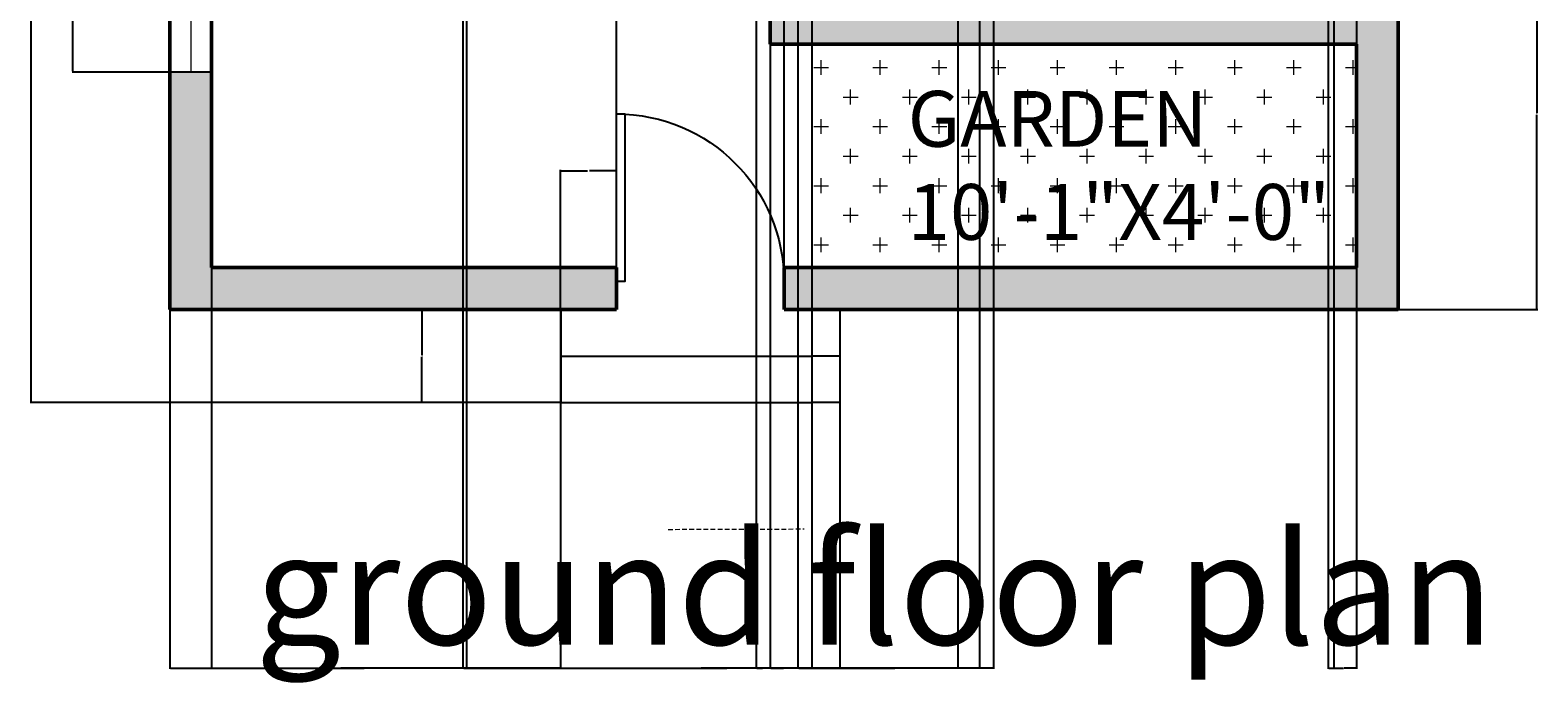
# Model space of a CAD drawing. Units: inches. Extents: x 1489 to 1813, y 1703 to 2293.
# Tile 1 of 4: x 1489 to 1813, y 1703 to 1843. Entities that reach past the tile are written whole.
import ezdxf

# ---------------------------------------------------------------- set-up
doc = ezdxf.new("R2010")
doc.units = ezdxf.units.IN
doc.header["$LTSCALE"] = 0.4
doc.linetypes.add('HIDDEN', pattern=[9.525, 6.35, -3.175])
for name, color, linetype, lineweight in [('A-ANNO-DIMS', 2, 'Continuous', 18), ('A-ANNO-HIDN', 7, 'HIDDEN', 18), ('A-ANNO-TEXT', 7, 'Continuous', 35), ('A-AREA-IDEN', 7, 'Continuous', 18), ('A-DOOR', 4, 'Continuous', 25), ('A-FLOR-STRS', 7, 'Continuous', 25), ('A-GLAZ', 4, 'Continuous', 18), ('A-WALL', 7, 'Continuous', 50), ('L-PLNT', 3, 'Continuous', 18)]:
    doc.layers.add(name, color=color, linetype=linetype, lineweight=lineweight)
doc.layers.add('A-WALL-PATT', color=18, linetype='HIDDEN', lineweight=13, true_color=0x000000)
doc.layers.add('L-PLNT-PATT', color=114, linetype='Continuous', lineweight=13, true_color=0x139b48)
doc.styles.get("Standard").update_dxf_attribs({"font": 'arial.ttf'})
doc.dimstyles.get("Standard").update_dxf_attribs({"dimtxt": 0.18, "dimasz": 0.18, "dimexe": 0.18, "dimexo": 0.0625, "dimgap": 0.09, "dimtad": 0, "dimtih": 1, "dimtoh": 1, "dimdec": 4, "dimzin": 0, "dimdsep": 46, "dimtxsty": 'Standard', "dimcen": 0.09, "dimadec": 0, "dimazin": 0, "dimtfac": 1, "dimtdec": 4, "dimtofl": 0, "dimtmove": 0, "dimatfit": 3, "dimfxl": 1, "dimtolj": 1, "dimtzin": 0, "dimarcsym": 0})

# ---------------------------------------------------------------- blocks, each defined once
blk = doc.blocks.new('*U5')
for p, q in [((-36, 0), (-36, -6)), ((0, 0), (0, -6))]:
    blk.add_line(p, q)
blk.add_lwpolyline([(0, 0), (0, 36), (-1.75, 36), (-1.75, 0)], close=True)
blk.add_arc((0, 0), 36, 90, 180)
blk = doc.blocks.new('*D29')
at = {"layer": 'A-ANNO-DIMS', "color": 0, "lineweight": -2, "ltscale": 0.4, "transparency": 16777216}
for p, q in [((1518.92, 2263.17), (1489, 2263.17)), ((1489.18, 2262.99), (1489.18, 2013.35)), ((1489.18, 1763.35), (1489.18, 2012.99)), ((1602.92, 1763.17), (1489, 1763.17))]:
    blk.add_line(p, q, dxfattribs=at)
at = {"layer": 'A-ANNO-DIMS', "color": 0, "ltscale": 0.4, "transparency": 16777216}
for points in [[(1489.15, 2262.99), (1489.21, 2262.99), (1489.18, 2263.17)], [(1489.15, 1763.35), (1489.21, 1763.35), (1489.18, 1763.17)]]:
    blk.add_solid(points, dxfattribs=at)
at = {"layer": 'Defpoints', "color": 0, "ltscale": 0.4, "transparency": 16777216}
for p in [(1489.18, 2263.17), (1518.98, 2263.17), (1602.98, 1763.17)]:
    blk.add_point(p, dxfattribs=at)
at = {"layer": 'A-ANNO-DIMS', "color": 0, "ltscale": 0.4, "transparency": 16777216, "insert": (1489.18, 2013.17), "char_height": 0.18, "attachment_point": 5}
blk.add_mtext('\\A1;500', dxfattribs=at)
blk = doc.blocks.new('*D30')
at = {"layer": 'A-ANNO-DIMS', "color": 0, "lineweight": -2, "ltscale": 0.4, "transparency": 16777216}
for p, q in [((1518.98, 1783.11), (1518.98, 1705.95)), ((1602.98, 1783.11), (1602.98, 1705.95)), ((1519.16, 1706.13), (1560.77, 1706.13)), ((1602.8, 1706.13), (1561.2, 1706.13))]:
    blk.add_line(p, q, dxfattribs=at)
at = {"layer": 'A-ANNO-DIMS', "color": 0, "ltscale": 0.4, "transparency": 16777216}
for points in [[(1519.16, 1706.16), (1519.16, 1706.1), (1518.98, 1706.13)], [(1602.8, 1706.16), (1602.8, 1706.1), (1602.98, 1706.13)]]:
    blk.add_solid(points, dxfattribs=at)
at = {"layer": 'Defpoints', "color": 0, "ltscale": 0.4, "transparency": 16777216}
for p in [(1518.98, 1783.17), (1602.98, 1783.17), (1602.98, 1706.13)]:
    blk.add_point(p, dxfattribs=at)
at = {"layer": 'A-ANNO-DIMS', "color": 0, "ltscale": 0.4, "transparency": 16777216, "insert": (1560.98, 1706.13), "char_height": 0.18, "attachment_point": 5}
blk.add_mtext('\\A1;84', dxfattribs=at)
blk = doc.blocks.new('*D31')
at = {"layer": 'A-ANNO-DIMS', "color": 0, "lineweight": -2, "ltscale": 0.4, "transparency": 16777216}
for p, q in [((1602.98, 1763.11), (1602.98, 1705.95)), ((1662.98, 1763.11), (1662.98, 1705.95)), ((1603.16, 1706.13), (1632.76, 1706.13)), ((1662.8, 1706.13), (1633.2, 1706.13))]:
    blk.add_line(p, q, dxfattribs=at)
at = {"layer": 'A-ANNO-DIMS', "color": 0, "ltscale": 0.4, "transparency": 16777216}
for points in [[(1603.16, 1706.16), (1603.16, 1706.1), (1602.98, 1706.13)], [(1662.8, 1706.16), (1662.8, 1706.1), (1662.98, 1706.13)]]:
    blk.add_solid(points, dxfattribs=at)
at = {"layer": 'Defpoints', "color": 0, "ltscale": 0.4, "transparency": 16777216}
for p in [(1602.98, 1763.17), (1662.98, 1763.17), (1662.98, 1706.13)]:
    blk.add_point(p, dxfattribs=at)
at = {"layer": 'A-ANNO-DIMS', "color": 0, "ltscale": 0.4, "transparency": 16777216, "insert": (1632.98, 1706.13), "char_height": 0.18, "attachment_point": 5}
blk.add_mtext('\\A1;60', dxfattribs=at)
blk = doc.blocks.new('*D32')
at = {"layer": 'A-ANNO-DIMS', "color": 0, "lineweight": -2, "ltscale": 0.4, "transparency": 16777216}
for p, q in [((1602.92, 1783.17), (1573, 1783.17)), ((1573.18, 1782.99), (1573.18, 1773.35)), ((1573.18, 1763.35), (1573.18, 1772.99)), ((1602.92, 1763.17), (1573, 1763.17))]:
    blk.add_line(p, q, dxfattribs=at)
at = {"layer": 'A-ANNO-DIMS', "color": 0, "ltscale": 0.4, "transparency": 16777216}
for points in [[(1573.15, 1782.99), (1573.21, 1782.99), (1573.18, 1783.17)], [(1573.15, 1763.35), (1573.21, 1763.35), (1573.18, 1763.17)]]:
    blk.add_solid(points, dxfattribs=at)
at = {"layer": 'Defpoints', "color": 0, "ltscale": 0.4, "transparency": 16777216}
for p in [(1573.18, 1783.17), (1602.98, 1783.17), (1602.98, 1763.17)]:
    blk.add_point(p, dxfattribs=at)
at = {"layer": 'A-ANNO-DIMS', "color": 0, "ltscale": 0.4, "transparency": 16777216, "insert": (1573.18, 1773.17), "char_height": 0.18, "attachment_point": 5}
blk.add_mtext('\\A1;20', dxfattribs=at)
blk = doc.blocks.new('*D33')
at = {"layer": 'A-ANNO-DIMS', "color": 0, "lineweight": -2, "ltscale": 0.4, "transparency": 16777216}
for p, q in [((1614.98, 1783.23), (1614.98, 2293.15)), ((1615.16, 2292.97), (1632.77, 2292.97)), ((1650.8, 2292.97), (1633.2, 2292.97)), ((1650.98, 1783.23), (1650.98, 2293.15))]:
    blk.add_line(p, q, dxfattribs=at)
at = {"layer": 'A-ANNO-DIMS', "color": 0, "ltscale": 0.4, "transparency": 16777216}
for points in [[(1615.16, 2293), (1615.16, 2292.94), (1614.98, 2292.97)], [(1650.8, 2293), (1650.8, 2292.94), (1650.98, 2292.97)]]:
    blk.add_solid(points, dxfattribs=at)
at = {"layer": 'Defpoints', "color": 0, "ltscale": 0.4, "transparency": 16777216}
for p in [(1650.98, 2292.97), (1614.98, 1783.17), (1650.98, 1783.17)]:
    blk.add_point(p, dxfattribs=at)
at = {"layer": 'A-ANNO-DIMS', "color": 0, "ltscale": 0.4, "transparency": 16777216, "insert": (1632.98, 2292.97), "char_height": 0.18, "attachment_point": 5}
blk.add_mtext('\\A1;36', dxfattribs=at)
blk = doc.blocks.new('*D34')
at = {"layer": 'A-ANNO-DIMS', "color": 0, "lineweight": -2, "ltscale": 0.4, "transparency": 16777216}
for p, q in [((1783.05, 1867.17), (1812.96, 1867.17)), ((1812.78, 1866.99), (1812.78, 1825.35)), ((1812.78, 1783.35), (1812.78, 1824.99)), ((1783.05, 1783.17), (1812.96, 1783.17))]:
    blk.add_line(p, q, dxfattribs=at)
at = {"layer": 'A-ANNO-DIMS', "color": 0, "ltscale": 0.4, "transparency": 16777216}
for points in [[(1812.75, 1866.99), (1812.81, 1866.99), (1812.78, 1867.17)], [(1812.75, 1783.35), (1812.81, 1783.35), (1812.78, 1783.17)]]:
    blk.add_solid(points, dxfattribs=at)
at = {"layer": 'Defpoints', "color": 0, "ltscale": 0.4, "transparency": 16777216}
for p in [(1782.98, 1867.17), (1812.78, 1867.17), (1782.98, 1783.17)]:
    blk.add_point(p, dxfattribs=at)
at = {"layer": 'A-ANNO-DIMS', "color": 0, "ltscale": 0.4, "transparency": 16777216, "insert": (1812.78, 1825.17), "char_height": 0.18, "attachment_point": 5}
blk.add_mtext('\\A1;84', dxfattribs=at)
blk = doc.blocks.new('*D41')
at = {"layer": 'A-ANNO-DIMS', "color": 0, "lineweight": -2, "ltscale": 0.4, "transparency": 16777216}
for p, q in [((1647.98, 2254.11), (1647.98, 1705.95)), ((1653.98, 2254.11), (1653.98, 1705.95)), ((1648.16, 1706.13), (1650.83, 1706.13)), ((1653.8, 1706.13), (1651.13, 1706.13))]:
    blk.add_line(p, q, dxfattribs=at)
at = {"layer": 'A-ANNO-DIMS', "color": 0, "ltscale": 0.4, "transparency": 16777216}
for points in [[(1648.16, 1706.16), (1648.16, 1706.1), (1647.98, 1706.13)], [(1653.8, 1706.16), (1653.8, 1706.1), (1653.98, 1706.13)]]:
    blk.add_solid(points, dxfattribs=at)
at = {"layer": 'Defpoints', "color": 0, "ltscale": 0.4, "transparency": 16777216}
for p in [(1647.98, 2254.17), (1653.98, 2254.17), (1653.98, 1706.13)]:
    blk.add_point(p, dxfattribs=at)
at = {"layer": 'A-ANNO-DIMS', "color": 0, "ltscale": 0.4, "transparency": 16777216, "insert": (1650.98, 1706.13), "char_height": 0.18, "attachment_point": 5}
blk.add_mtext('\\A1;6', dxfattribs=at)
blk = doc.blocks.new('*D42')
at = {"layer": 'A-ANNO-DIMS', "color": 0, "lineweight": -2, "ltscale": 0.4, "transparency": 16777216}
for p, q in [((1527.92, 1882.17), (1498, 1882.17)), ((1498.18, 1881.99), (1498.18, 1858.35)), ((1498.18, 1834.35), (1498.18, 1857.99)), ((1527.92, 1834.17), (1498, 1834.17))]:
    blk.add_line(p, q, dxfattribs=at)
at = {"layer": 'A-ANNO-DIMS', "color": 0, "ltscale": 0.4, "transparency": 16777216}
for points in [[(1498.15, 1881.99), (1498.21, 1881.99), (1498.18, 1882.17)], [(1498.15, 1834.35), (1498.21, 1834.35), (1498.18, 1834.17)]]:
    blk.add_solid(points, dxfattribs=at)
at = {"layer": 'Defpoints', "color": 0, "ltscale": 0.4, "transparency": 16777216}
for p in [(1498.18, 1882.17), (1527.98, 1882.17), (1527.98, 1834.17)]:
    blk.add_point(p, dxfattribs=at)
at = {"layer": 'A-ANNO-DIMS', "color": 0, "ltscale": 0.4, "transparency": 16777216, "insert": (1498.18, 1858.17), "char_height": 0.18, "attachment_point": 5}
blk.add_mtext('\\A1;48', dxfattribs=at)
blk = doc.blocks.new('*D52')
at = {"layer": 'A-ANNO-DIMS', "color": 0, "lineweight": -2, "ltscale": 0.4, "transparency": 16777216}
for p, q in [((1527.98, 2254.11), (1527.98, 1705.95)), ((1582.71, 2254.11), (1582.71, 1705.95)), ((1528.16, 1706.13), (1554.95, 1706.13)), ((1582.53, 1706.13), (1555.74, 1706.13))]:
    blk.add_line(p, q, dxfattribs=at)
at = {"layer": 'A-ANNO-DIMS', "color": 0, "ltscale": 0.4, "transparency": 16777216}
for points in [[(1528.16, 1706.16), (1528.16, 1706.1), (1527.98, 1706.13)], [(1582.53, 1706.16), (1582.53, 1706.1), (1582.71, 1706.13)]]:
    blk.add_solid(points, dxfattribs=at)
at = {"layer": 'Defpoints', "color": 0, "ltscale": 0.4, "transparency": 16777216}
for p in [(1527.98, 2254.17), (1582.71, 2254.17), (1582.71, 1706.13)]:
    blk.add_point(p, dxfattribs=at)
at = {"layer": 'A-ANNO-DIMS', "color": 0, "ltscale": 0.4, "transparency": 16777216, "insert": (1555.35, 1706.13), "char_height": 0.18, "attachment_point": 5}
blk.add_mtext('\\A1;54.73', dxfattribs=at)
blk = doc.blocks.new('*D53')
at = {"layer": 'A-ANNO-DIMS', "color": 0, "lineweight": -2, "ltscale": 0.4, "transparency": 16777216}
for p, q in [((1656.98, 2122.11), (1656.98, 1705.95)), ((1692.98, 2122.11), (1692.98, 1705.95)), ((1657.16, 1706.13), (1674.77, 1706.13)), ((1692.8, 1706.13), (1675.2, 1706.13))]:
    blk.add_line(p, q, dxfattribs=at)
at = {"layer": 'A-ANNO-DIMS', "color": 0, "ltscale": 0.4, "transparency": 16777216}
for points in [[(1657.16, 1706.16), (1657.16, 1706.1), (1656.98, 1706.13)], [(1692.8, 1706.16), (1692.8, 1706.1), (1692.98, 1706.13)]]:
    blk.add_solid(points, dxfattribs=at)
at = {"layer": 'Defpoints', "color": 0, "ltscale": 0.4, "transparency": 16777216}
for p in [(1656.98, 2122.17), (1692.98, 2122.17), (1692.98, 1706.13)]:
    blk.add_point(p, dxfattribs=at)
at = {"layer": 'A-ANNO-DIMS', "color": 0, "ltscale": 0.4, "transparency": 16777216, "insert": (1674.98, 1706.13), "char_height": 0.18, "attachment_point": 5}
blk.add_mtext('\\A1;36', dxfattribs=at)
blk = doc.blocks.new('*D56')
at = {"layer": 'A-ANNO-DIMS', "color": 0, "lineweight": -2, "ltscale": 0.4, "transparency": 16777216}
for p, q in [((1602.98, 1783.23), (1602.98, 1813.15)), ((1603.16, 1812.97), (1608.77, 1812.97)), ((1614.8, 1812.97), (1609.19, 1812.97)), ((1614.98, 1783.23), (1614.98, 1813.15))]:
    blk.add_line(p, q, dxfattribs=at)
at = {"layer": 'A-ANNO-DIMS', "color": 0, "ltscale": 0.4, "transparency": 16777216}
for points in [[(1603.16, 1813), (1603.16, 1812.94), (1602.98, 1812.97)], [(1614.8, 1813), (1614.8, 1812.94), (1614.98, 1812.97)]]:
    blk.add_solid(points, dxfattribs=at)
at = {"layer": 'Defpoints', "color": 0, "ltscale": 0.4, "transparency": 16777216}
for p in [(1614.98, 1812.97), (1602.98, 1783.17), (1614.98, 1783.17)]:
    blk.add_point(p, dxfattribs=at)
at = {"layer": 'A-ANNO-DIMS', "color": 0, "ltscale": 0.4, "transparency": 16777216, "insert": (1608.98, 1812.97), "char_height": 0.18, "attachment_point": 5}
blk.add_mtext('\\A1;12', dxfattribs=at)
blk = doc.blocks.new('*D57')
at = {"layer": 'A-ANNO-DIMS', "color": 0, "lineweight": -2, "ltscale": 0.4, "transparency": 16777216}
for p, q in [((1644.98, 1930.11), (1644.98, 1705.95)), ((1647.98, 1930.11), (1647.98, 1705.95)), ((1645.16, 1706.13), (1646.33, 1706.13)), ((1647.8, 1706.13), (1646.63, 1706.13))]:
    blk.add_line(p, q, dxfattribs=at)
at = {"layer": 'A-ANNO-DIMS', "color": 0, "ltscale": 0.4, "transparency": 16777216}
for points in [[(1645.16, 1706.16), (1645.16, 1706.1), (1644.98, 1706.13)], [(1647.8, 1706.16), (1647.8, 1706.1), (1647.98, 1706.13)]]:
    blk.add_solid(points, dxfattribs=at)
at = {"layer": 'Defpoints', "color": 0, "ltscale": 0.4, "transparency": 16777216}
for p in [(1644.98, 1930.17), (1647.98, 1930.17), (1647.98, 1706.13)]:
    blk.add_point(p, dxfattribs=at)
at = {"layer": 'A-ANNO-DIMS', "color": 0, "ltscale": 0.4, "transparency": 16777216, "insert": (1646.48, 1706.13), "char_height": 0.18, "attachment_point": 5}
blk.add_mtext('\\A1;3', dxfattribs=at)
blk = doc.blocks.new('*D59')
at = {"layer": 'A-ANNO-DIMS', "color": 0, "lineweight": -2, "ltscale": 0.4, "transparency": 16777216}
for p, q in [((1653.98, 2254.11), (1653.98, 1705.95)), ((1688.31, 2248.43), (1688.31, 1705.95)), ((1654.16, 1706.13), (1670.75, 1706.13)), ((1688.13, 1706.13), (1671.54, 1706.13))]:
    blk.add_line(p, q, dxfattribs=at)
at = {"layer": 'A-ANNO-DIMS', "color": 0, "ltscale": 0.4, "transparency": 16777216}
for points in [[(1654.16, 1706.16), (1654.16, 1706.1), (1653.98, 1706.13)], [(1688.13, 1706.16), (1688.13, 1706.1), (1688.31, 1706.13)]]:
    blk.add_solid(points, dxfattribs=at)
at = {"layer": 'Defpoints', "color": 0, "ltscale": 0.4, "transparency": 16777216}
for p in [(1653.98, 2254.17), (1688.31, 2248.49), (1688.31, 1706.13)]:
    blk.add_point(p, dxfattribs=at)
at = {"layer": 'A-ANNO-DIMS', "color": 0, "ltscale": 0.4, "transparency": 16777216, "insert": (1671.14, 1706.13), "char_height": 0.18, "attachment_point": 5}
blk.add_mtext('\\A1;34.32', dxfattribs=at)
blk = doc.blocks.new('*D61')
at = {"layer": 'A-ANNO-DIMS', "color": 0, "lineweight": -2, "ltscale": 0.4, "transparency": 16777216}
for p, q in [((1773.98, 2050.11), (1773.98, 1705.95)), ((1769.14, 2025.11), (1769.14, 1705.95)), ((1769.32, 1706.13), (1771.17, 1706.13)), ((1773.8, 1706.13), (1771.96, 1706.13))]:
    blk.add_line(p, q, dxfattribs=at)
at = {"layer": 'A-ANNO-DIMS', "color": 0, "ltscale": 0.4, "transparency": 16777216}
for points in [[(1769.32, 1706.16), (1769.32, 1706.1), (1769.14, 1706.13)], [(1773.8, 1706.16), (1773.8, 1706.1), (1773.98, 1706.13)]]:
    blk.add_solid(points, dxfattribs=at)
at = {"layer": 'Defpoints', "color": 0, "ltscale": 0.4, "transparency": 16777216}
for p in [(1773.98, 2050.17), (1769.14, 2025.17), (1773.98, 1706.13)]:
    blk.add_point(p, dxfattribs=at)
at = {"layer": 'A-ANNO-DIMS', "color": 0, "ltscale": 0.4, "transparency": 16777216, "insert": (1771.56, 1706.13), "char_height": 0.18, "attachment_point": 5}
blk.add_mtext('\\A1;4.844', dxfattribs=at)
blk = doc.blocks.new('*D63')
at = {"layer": 'A-ANNO-DIMS', "color": 0, "lineweight": -2, "ltscale": 0.4, "transparency": 16777216}
for p, q in [((1581.98, 2062.11), (1581.98, 1705.95)), ((1695.98, 2056.11), (1695.98, 1705.95)), ((1582.16, 1706.13), (1638.7, 1706.13)), ((1695.8, 1706.13), (1639.26, 1706.13))]:
    blk.add_line(p, q, dxfattribs=at)
at = {"layer": 'A-ANNO-DIMS', "color": 0, "ltscale": 0.4, "transparency": 16777216}
for points in [[(1582.16, 1706.16), (1582.16, 1706.1), (1581.98, 1706.13)], [(1695.8, 1706.16), (1695.8, 1706.1), (1695.98, 1706.13)]]:
    blk.add_solid(points, dxfattribs=at)
at = {"layer": 'Defpoints', "color": 0, "ltscale": 0.4, "transparency": 16777216}
for p in [(1581.98, 2062.17), (1695.98, 2056.17), (1695.98, 1706.13)]:
    blk.add_point(p, dxfattribs=at)
at = {"layer": 'A-ANNO-DIMS', "color": 0, "ltscale": 0.4, "transparency": 16777216, "insert": (1638.98, 1706.13), "char_height": 0.18, "attachment_point": 5}
blk.add_mtext('\\A1;114', dxfattribs=at)
blk = doc.blocks.new('*D64')
at = {"layer": 'A-ANNO-DIMS', "color": 0, "lineweight": -2, "ltscale": 0.4, "transparency": 16777216}
for p, q in [((1767.89, 2061.85), (1767.89, 1705.95)), ((1773.98, 2056.11), (1773.98, 1705.95)), ((1768.07, 1706.13), (1770.56, 1706.13)), ((1773.8, 1706.13), (1771.31, 1706.13))]:
    blk.add_line(p, q, dxfattribs=at)
at = {"layer": 'A-ANNO-DIMS', "color": 0, "ltscale": 0.4, "transparency": 16777216}
for points in [[(1768.07, 1706.16), (1768.07, 1706.1), (1767.89, 1706.13)], [(1773.8, 1706.16), (1773.8, 1706.1), (1773.98, 1706.13)]]:
    blk.add_solid(points, dxfattribs=at)
at = {"layer": 'Defpoints', "color": 0, "ltscale": 0.4, "transparency": 16777216}
for p in [(1767.89, 2061.91), (1773.98, 2056.17), (1773.98, 1706.13)]:
    blk.add_point(p, dxfattribs=at)
at = {"layer": 'A-ANNO-DIMS', "color": 0, "ltscale": 0.4, "transparency": 16777216, "insert": (1770.94, 1706.13), "char_height": 0.18, "attachment_point": 5}
blk.add_mtext('\\A1;6.091', dxfattribs=at)

msp = doc.modelspace()

# ---------------------------------------------------------------- hatches: boundary and pattern name
at = {"layer": 'A-WALL-PATT', "ltscale": 0.4}
h = msp.add_hatch(dxfattribs=at)
h.set_pattern_fill('HONEY', color=256, scale=0.1)
h.paths.add_polyline_path([(1527.9839, 2128.1709), (1575.9839, 2128.1709), (1575.9839, 2125.1709), (1581.9839, 2125.1709), (1581.9839, 2134.1709), (1527.9839, 2134.1709), (1527.9839, 2170.1709), (1518.9839, 2170.1709), (1518.9839, 2020.1709), (1527.9839, 2020.1709), (1527.9839, 2062.1709), (1581.9839, 2062.1709), (1581.9839, 2095.1709), (1575.9839, 2095.1709), (1575.9839, 2068.1709), (1527.9839, 2068.1709)])
h.paths.add_polyline_path([(1527.9839, 1924.1709), (1608.9839, 1924.1709), (1608.9839, 1930.1709), (1527.9839, 1930.1709), (1527.9839, 1972.1709), (1518.9839, 1972.1709), (1518.9839, 1882.1709), (1527.9839, 1882.1709)])
h.paths.add_polyline_path([(1527.9839, 1834.1709), (1518.9839, 1834.1709), (1518.9839, 1783.1709), (1614.9839, 1783.1709), (1614.9839, 1789.1709), (1614.9839, 1792.1709), (1527.9839, 1792.1709)])
h.paths.add_polyline_path([(1782.9839, 1867.1709), (1773.9839, 1867.1709), (1773.9839, 1846.1709), (1647.9839, 1846.1709), (1647.9839, 1840.1709), (1773.9839, 1840.1709), (1773.9839, 1792.1709), (1650.9839, 1792.1709), (1650.9839, 1783.1709), (1782.9839, 1783.1709)])
h.paths.add_polyline_path([(1540.5005, 2064.0337), (1577.6874, 2064.0337), (1577.6874, 2090.1253), (1540.5005, 2090.1253)], flags=24)
at = {"layer": 'L-PLNT-PATT'}
h = msp.add_hatch(dxfattribs=at)
h.set_pattern_fill('CROSS', color=256)
h.paths.add_polyline_path([(1773.9839, 1840.1709), (1653.9839, 1840.1709), (1653.9839, 1792.1709), (1773.9839, 1792.1709)])

# ---------------------------------------------------------------- linework, layer by layer
at = {"layer": 'A-ANNO-HIDN', "ltscale": 0.4}
msp.add_line((1626.053, 1735.9265), (1655.3291, 1736.0155), dxfattribs=at)
at = {"layer": 'A-FLOR-STRS'}
for p, q in [((1614.9839, 1783.1709), (1602.9839, 1783.1709)), ((1602.9839, 1783.1709), (1602.9839, 1773.1709)), ((1650.9839, 1783.1709), (1662.9839, 1783.1709)), ((1662.9839, 1783.1709), (1662.9839, 1773.1709)), ((1602.9839, 1773.1709), (1657.0024, 1773.1709)), ((1602.9839, 1773.1709), (1602.9839, 1763.1709)), ((1662.9839, 1773.1709), (1657.0024, 1773.1709)), ((1662.9839, 1773.1709), (1662.9839, 1763.1709)), ((1602.9839, 1763.1709), (1657.0024, 1763.1709)), ((1662.9839, 1763.1709), (1657.0024, 1763.1709))]:
    msp.add_line(p, q, dxfattribs=at)
at = {"layer": 'A-GLAZ'}
for p, q in [((1523.4839, 1882.1709), (1523.4839, 1834.1709)), ((1527.9839, 1834.1709), (1518.9839, 1834.1709))]:
    msp.add_line(p, q, dxfattribs=at)
at = {"layer": 'A-WALL'}
for p, q in [((1518.9839, 2263.1709), (1518.9839, 1783.1709)), ((1782.9839, 1783.1709), (1782.9839, 2263.1709)), ((1527.9839, 1924.1709), (1527.9839, 1792.1709)), ((1647.9839, 1846.1709), (1647.9839, 1840.1709)), ((1647.9839, 1840.1709), (1773.9839, 1840.1709)), ((1773.9839, 1792.1709), (1773.9839, 1840.1709)), ((1527.9839, 1792.1709), (1614.9839, 1792.1709)), ((1614.9839, 1792.1709), (1614.9839, 1783.1709)), ((1650.9839, 1792.1709), (1650.9839, 1783.1709)), ((1650.9839, 1792.1709), (1773.9839, 1792.1709)), ((1518.9839, 1783.1709), (1614.9839, 1783.1709)), ((1650.9839, 1783.1709), (1782.9839, 1783.1709))]:
    msp.add_line(p, q, dxfattribs=at)
at = {"layer": 'L-PLNT'}
for p, q in [((1653.9839, 1792.1709), (1653.9839, 1840.1709)), ((1653.9839, 1840.1709), (1653.9839, 1792.1709))]:
    msp.add_line(p, q, dxfattribs=at)

# ---------------------------------------------------------------- block references
at = {"layer": 'A-DOOR', "xscale": -1}
msp.add_blockref('*U5', (1614.9839, 1789.1709), dxfattribs=at)

# ---------------------------------------------------------------- texts
at = {"layer": 'A-ANNO-TEXT', "insert": (1537.3049, 1735.1422), "char_height": 24, "attachment_point": 1}
msp.add_mtext_dynamic_manual_height_columns('ground floor plan ', width=497.197095, gutter_width=12.5, heights=[0], dxfattribs=at)
at = {"layer": 'A-AREA-IDEN', "insert": (1677.5571, 1830.1247), "char_height": 12, "attachment_point": 1}
msp.add_mtext_dynamic_manual_height_columns('GARDEN\\P10\'-1"X4\'-0"', width=79.191819, gutter_width=12.5, heights=[0], dxfattribs=at)

# ---------------------------------------------------------------- dimensions: what is measured, and where the dimension line sits
at = {"layer": 'A-ANNO-DIMS', "ltscale": 0.4}
for base, p1, p2, override, picture, middle in [((1650.9839, 2292.9709), (1614.9839, 1783.1709), (1650.9839, 1783.1709), {"dimdec": 0, "dimlfac": 1, "dimrnd": 0, "dimzin": 0, "dimdsep": 46, "dimlunit": 2}, '*D33', (1632.9839, 2292.9709)), ((1582.7115, 1706.1265), (1527.9839, 2254.1709), (1582.7115, 2254.1709), {"dimdec": 2, "dimlfac": 1, "dimrnd": 0, "dimzin": 0, "dimdsep": 46, "dimlunit": 2}, '*D52', (1555.3477, 1706.1265)), ((1653.9839, 1706.1265), (1647.9839, 2254.1709), (1653.9839, 2254.1709), {"dimdec": 0, "dimlfac": 1, "dimrnd": 0, "dimzin": 0, "dimdsep": 46, "dimlunit": 2}, '*D41', (1650.9839, 1706.1265)), ((1688.3051, 1706.1265), (1653.9839, 2254.1709), (1688.3051, 2248.4927), {"dimdec": 2, "dimlfac": 1, "dimrnd": 0, "dimzin": 0, "dimdsep": 46, "dimlunit": 2}, '*D59', (1671.1445, 1706.1265)), ((1692.9839, 1706.1265), (1656.9839, 2122.1709), (1692.9839, 2122.1709), {"dimdec": 0, "dimlfac": 1, "dimrnd": 0, "dimzin": 0, "dimdsep": 46, "dimlunit": 2}, '*D53', (1674.9839, 1706.1265)), ((1695.9839, 1706.1265), (1581.9839, 2062.1709), (1695.9839, 2056.1709), {"dimdec": 0, "dimlfac": 1, "dimrnd": 0, "dimzin": 0, "dimdsep": 46, "dimlunit": 2}, '*D63', (1638.9839, 1706.1265)), ((1773.98388, 1706.12655), (1767.89245, 2061.91042), (1773.98388, 2056.17088), {"dimdec": 3, "dimlfac": 1, "dimrnd": 0, "dimzin": 0, "dimdsep": 46, "dimlunit": 2}, '*D64', (1770.93817, 1706.12655)), ((1773.9839, 1706.1265), (1769.1403, 2025.1698), (1773.9839, 2050.1709), {"dimdec": 3, "dimlfac": 1, "dimrnd": 0, "dimzin": 0, "dimdsep": 46, "dimlunit": 2}, '*D61', (1771.5621, 1706.1265)), ((1647.9839, 1706.1265), (1644.9839, 1930.1709), (1647.9839, 1930.1709), {"dimdec": 0, "dimlfac": 1, "dimrnd": 0, "dimzin": 0, "dimdsep": 46, "dimlunit": 2}, '*D57', (1646.4839, 1706.1265)), ((1614.9839, 1812.9709), (1602.9839, 1783.1709), (1614.9839, 1783.1709), {"dimdec": 0, "dimlfac": 1, "dimrnd": 0, "dimzin": 0, "dimdsep": 46, "dimlunit": 2}, '*D56', (1608.9839, 1812.9709)), ((1602.9839, 1706.1265), (1518.9839, 1783.1709), (1602.9839, 1783.1709), {"dimdec": 0, "dimlfac": 1, "dimrnd": 0, "dimzin": 0, "dimdsep": 46, "dimlunit": 2}, '*D30', (1560.9839, 1706.1265)), ((1662.9839, 1706.1265), (1602.9839, 1763.1709), (1662.9839, 1763.1709), {"dimdec": 0, "dimlfac": 1, "dimrnd": 0, "dimzin": 0, "dimdsep": 46, "dimlunit": 2}, '*D31', (1632.9839, 1706.1265))]:
    dim = msp.add_linear_dim(base=base, p1=p1, p2=p2, dimstyle='Standard', override=override, dxfattribs=at)
    dim.commit()
    dim.dimension.update_dxf_attribs({"geometry": picture, "text_midpoint": middle})
for base, p1, p2, picture, middle in [((1489.1839, 2263.1709), (1602.9839, 1763.1709), (1518.9839, 2263.1709), '*D29', (1489.1839, 2013.1709)), ((1498.1839, 1882.1709), (1527.9839, 1834.1709), (1527.9839, 1882.1709), '*D42', (1498.1839, 1858.1709)), ((1812.7839, 1867.1709), (1782.9839, 1783.1709), (1782.9839, 1867.1709), '*D34', (1812.7839, 1825.1709)), ((1573.1839, 1783.1709), (1602.9839, 1763.1709), (1602.9839, 1783.1709), '*D32', (1573.1839, 1773.1709))]:
    dim = msp.add_linear_dim(base=base, p1=p1, p2=p2, angle=90, dimstyle='Standard', override={"dimdec": 0, "dimlfac": 1, "dimrnd": 0, "dimzin": 0, "dimdsep": 46, "dimlunit": 2}, dxfattribs=at)
    dim.commit()
    dim.dimension.update_dxf_attribs({"geometry": picture, "text_midpoint": middle})

doc.saveas('drawing.dxf')
